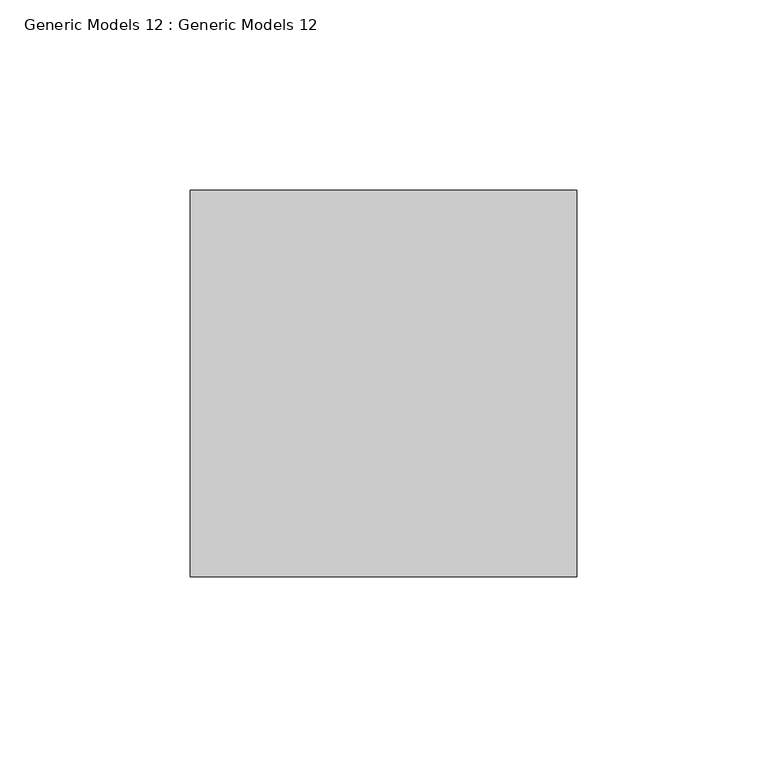
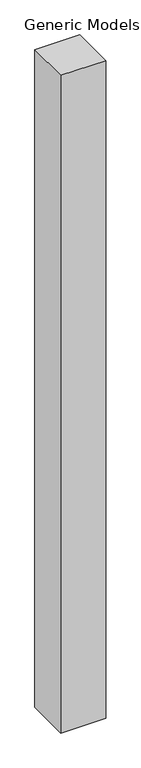
"""IFC4 building model written with IfcOpenShell, lengths in millimetres: proxy geometry, Generic Models 12 : Generic Models 12."""

from ifc_helpers import new_model, si_unit, frame, origin, place, context, project, spatial, polyline, outline, extrude, source, transform, mapped, element, save


def generic_models_12_generic_models_12_14ee2a94(model_context):
    return source(origin(), model_context, "Body", "SweptSolid", [
        extrude(outline(polyline([(-10607.7857944, -3188.4825197), (-10607.7857944, -3290.0825197), (-10709.3857944, -3290.0825197), (-10709.3857944, -3188.4825197), (-10607.7857944, -3188.4825197)])), frame((0.0, 0.0, 1524.0), z_axis=(0.0, 0.0, 1.0), x_axis=(1.0, 0.0, 0.0)), (0.0, 0.0, 1.0), 1574.8),
    ])


if __name__ == "__main__":
    model = new_model("IFC4")
    model_context = context("Model", 3, world=origin())
    ifc_project = project(units=[si_unit("LENGTHUNIT", "METRE", prefix="MILLI")], contexts=[model_context])
    site = spatial("IfcSite", under=ifc_project)
    building = spatial("IfcBuilding", under=site)
    placement = place(None, origin())
    generic_models_12_generic_models_12_shape = generic_models_12_generic_models_12_14ee2a94(model_context)
    element("IfcBuildingElementProxy", 1, Name="Generic Models 12 : Generic Models 12", ObjectType="Generic Models 12 : Generic Models 12", at=placement, inside=building, context=model_context, shape_type="MappedRepresentation", body=[
        mapped(generic_models_12_generic_models_12_shape, transform((0.0, 0.0, 0.0), x_axis=(1.0, 0.0, 0.0), y_axis=(0.0, 1.0, 0.0), z_axis=(0.0, 0.0, 1.0))),
    ])
    save(model, "model.ifc")

# Revit data of these elements
# Element 1 (IfcBuildingElementProxy, "Generic Models 12 : Generic Models 12")
#   Materials on its faces: "Steel, Carbon"
# Materials
#   "Steel, Carbon": class "Metal", colour RGB 0 0 0, transparency 0, Description = "Carbon steel", Cost = 0
